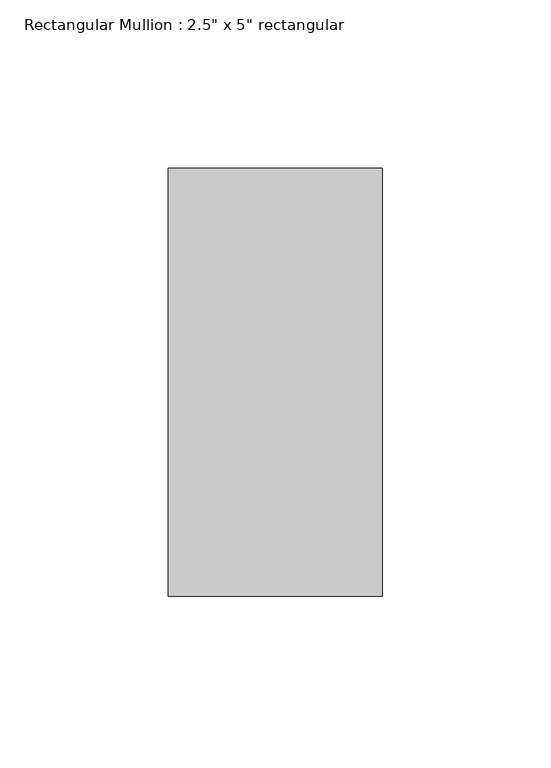
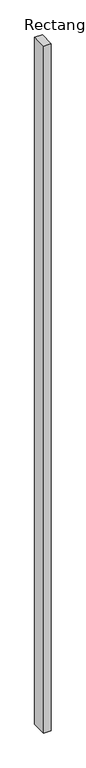
"""IFC4 building model written with IfcOpenShell, lengths in millimetres: member geometry."""

from ifc_helpers import new_model, si_unit, frame, origin, place, context, project, spatial, polyline, outline, extrude, source, transform, mapped, element, save


def member_74cc3c14(model_context):
    return source(origin(), model_context, "Body", "SweptSolid", [
        extrude(outline(polyline([(0.0, 63.5), (0.0, -63.5), (-63.5, -63.5), (-63.5, 63.5), (0.0, 63.5)])), frame((0.0, 0.0, -6000.7551516), z_axis=(0.0, 0.0, 1.0), x_axis=(1.0, 0.0, 0.0)), (0.0, 0.0, 1.0), 6000.7551516),
    ])


if __name__ == "__main__":
    model = new_model("IFC4")
    model_context = context("Model", 3, world=origin())
    ifc_project = project(units=[si_unit("LENGTHUNIT", "METRE", prefix="MILLI")], contexts=[model_context])
    site = spatial("IfcSite", under=ifc_project)
    building = spatial("IfcBuilding", under=site)
    placement = place(None, origin())
    member_shape = member_74cc3c14(model_context)
    element("IfcMember", 1, ObjectType="Rectangular Mullion : 2.5\" x 5\" rectangular", at=placement, inside=building, context=model_context, shape_type="MappedRepresentation", body=[
        mapped(member_shape, transform((0.0, 0.0, 0.0), x_axis=(1.0, 0.0, 0.0), y_axis=(0.0, 1.0, 0.0), z_axis=(0.0, 0.0, 1.0))),
    ])
    save(model, "model.ifc")

# Revit data of these elements
# Type "Rectangular Mullion : 2.5\" x 5\" rectangular"
#   built-in parameter 1007304 = 0.416667 (stored number, unit not read)
#   built-in parameter 1007301 = 0.104167 (stored number, unit not read)
#   built-in parameter 1007300 = 0.104167 (stored number, unit not read)
# Element 1 (IfcMember, "Rectangular Mullion : 2.5\" x 5\" rectangular")
#   Materials on its faces: "Iron, Ductile"
# Materials
#   "Iron, Ductile": class "Metal", colour RGB 0 0 0, transparency 0, Description = "Ductile cast iron", Cost = 0
